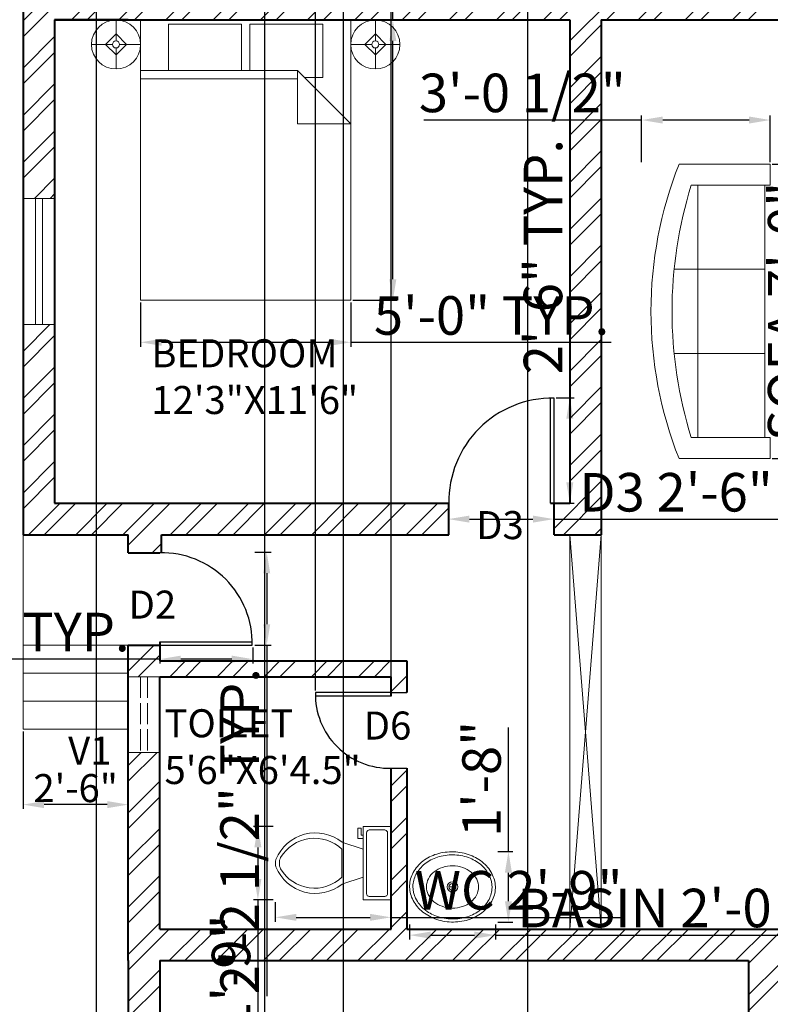
# Model space of a CAD drawing. Units: inches. Extents: x 2069 to 3028, y 691 to 1726.
# Tile 4 of 10: x 2267 to 2481, y 1044 to 1325. Entities that reach past the tile are written whole.
import ezdxf

# ---------------------------------------------------------------- set-up
doc = ezdxf.new("R2010")
doc.units = ezdxf.units.IN
doc.linetypes.add('ACAD_ISO02W100', pattern=[15, 12, -3])
for name, color, linetype, lineweight in [('A-ANNO-DIMS', 2, 'Continuous', 18), ('A-DOOR', 3, 'Continuous', 25), ('A-FLOR-FIXT', 9, 'Continuous', 20), ('A-FLOR-STRS', 7, 'Continuous', 20), ('A-FURN', 8, 'Continuous', 18), ('A-GLAZ', 4, 'Continuous', 20), ('A-GLAZ-HIDN', 4, 'ACAD_ISO02W100', 18), ('A-WALL', 7, 'Continuous', 40)]:
    doc.layers.add(name, color=color, linetype=linetype, lineweight=lineweight)
for name, color, linetype, lineweight, true_color in [('A-ANNO-TEXT', 11, 'Continuous', 18, 0xf27172), ('A-AREA-IDEN', 11, 'Continuous', 25, 0xf27172), ('A-WALL-OPEN', 143, 'Continuous', 20, 0x7aafdf), ('A-WALL-PATT', 143, 'Continuous', 13, 0x7aafdf)]:
    doc.layers.add(name, color=color, linetype=linetype, lineweight=lineweight, true_color=true_color)
doc.styles.get("Standard").update_dxf_attribs({"font": 'arial.ttf'})
doc.dimstyles.new('ISO-25', dxfattribs={"dimtxt": 11, "dimasz": 6, "dimexe": 1.25, "dimexo": 0.625, "dimtad": 1, "dimlunit": 3, "dimtxsty": 'Standard', "dimcen": 2.5, "dimclrd": 3, "dimclre": 5, "dimclrt": 6, "dimadec": 0, "dimazin": 0, "dimtfac": 1, "dimtmove": 0, "dimatfit": 3, "dimfxl": 1, "dimarcsym": 0})

# ---------------------------------------------------------------- blocks, each defined once
blk = doc.blocks.new('Sink - Oval top')
for p, q in [((-1, 0), (1, 0)), ((0, 1), (0, -1))]:
    blk.add_line(p, q)
for points in [[(-12.23, 0.39, 0.117634), (-11.46, -3.36, 0.104469), (-8.88, -6.8, 0.090016), (-5.08, -9.07, 0.08192), (-0.32, -10.02, 0.08192), (4.49, -9.38, 0.090016), (8.42, -7.36, 0.104469), (11.22, -4.09, 0.117634), (12.23, -0.39, 0.117634), (11.46, 3.36, 0.104469), (8.88, 6.8, 0.090016), (5.08, 9.07, 0.08192), (0.32, 10.02, 0.08192), (-4.49, 9.38, 0.090016), (-8.42, 7.36, 0.104469), (-11.22, 4.09, 0.117634)], [(-11.29, 0.16, 0.118622), (-10.52, -3.25, 0.104678), (-8.07, -6.36, 0.089562), (-4.54, -8.37, 0.081185), (-0.13, -9.15, 0.081185), (4.3, -8.49, 0.089562), (7.89, -6.58, 0.104678), (10.42, -3.55, 0.118622), (11.29, -0.16, 0.118622), (10.52, 3.25, 0.104678), (8.07, 6.36, 0.089562), (4.54, 8.37, 0.081185), (0.13, 9.15, 0.081185), (-4.3, 8.49, 0.089562), (-7.89, 6.58, 0.104678), (-10.42, 3.55, 0.118622)], [(-7.42, 0.08, 0.118283), (-6.91, -2.17, 0.104607), (-5.29, -4.21, 0.089718), (-2.97, -5.53, 0.081436), (-0.07, -6.04, 0.081436), (2.84, -5.59, 0.089718), (5.2, -4.33, 0.104607), (6.86, -2.32, 0.118283), (7.42, -0.08, 0.118283), (6.91, 2.17, 0.104607), (5.29, 4.21, 0.089718), (2.97, 5.53, 0.081436), (0.07, 6.04, 0.081436), (-2.84, 5.59, 0.089718), (-5.2, 4.33, 0.104607), (-6.86, 2.32, 0.118283)]]:
    blk.add_lwpolyline(points, format="xyb", close=True)
for radius in [1.5, 1]:
    blk.add_circle((0, 0), radius)
blk = doc.blocks.new('Bed - Queen')
for p, q in [((0, -80.00003), (0, 0)), ((0, 0), (59.99999, 0)), ((59.99999, 0), (59.99999, -80.00003)), ((7.99999, -1.2), (28.79998, -1.2)), ((7.99999, -14.4), (7.99999, -1.2)), ((28.79998, -1.2), (28.79998, -14.4)), ((31.19999, -1.2), (51.99999, -1.2)), ((31.19999, -14.4), (31.19999, -1.2)), ((51.99999, -1.2), (51.99999, -16.4)), ((0, -14.4), (44.8, -14.4)), ((44.8, -16.8), (0, -16.8)), ((59.99999, -29.6), (44.8, -14.4)), ((44.8, -14.4), (44.8, -29.6)), ((51.99999, -16.4), (46.79936, -16.4)), ((44.8, -29.6), (59.99999, -29.6)), ((59.99999, -80.00003), (0, -80.00003))]:
    blk.add_line(p, q)
blk = doc.blocks.new('Lamp - Table')
for p, q in [((0, 7), (0, 1)), ((0, 3), (-3, 0)), ((3, 0), (0, 3)), ((-1, 0), (-7, 0)), ((-3, 0), (0, -3)), ((0, -3), (3, 0)), ((1, 0), (7, 0)), ((0, -1), (0, -7))]:
    blk.add_line(p, q)
for radius in [7, 1]:
    blk.add_circle((0, 0), radius)
blk = doc.blocks.new('Sofa - Roundback 7 ft.')
for p, q in [((-12.00002, -32.4421), (-12.00003, -6.5971)), ((11.99997, -32.4421), (11.99998, -6.5971)), ((-36.000027, -34), (-36.000027, -11.4696)), ((-35.999844, -13.3819), (35.9998, -13.3819)), ((35.99998, -34), (35.99998, -11.4696)), ((-36.000027, -32.4421), (35.99998, -32.4421))]:
    blk.add_line(p, q)
for points in [[(-36.000027, -34), (-42.000027, -34), (-42.000027, -8)], [(41.99998, -8), (41.99998, -34), (35.99998, -34)]]:
    blk.add_lwpolyline(points)
for centre, radius, start, end in [((0, -114.25), 114.25, 68.43141, 111.5686), ((-0.00001, -127.1968), 121.1968, 72.72033, 107.2797)]:
    blk.add_arc(centre, radius, start, end)
blk = doc.blocks.new('Toilet - top')
for p, q in [((9.5, -6), (9.5, -2)), ((-8, -8.5), (-8, -8)), ((-7, -8), (-7, -9.5)), ((-4, -8), (-6, -14)), ((4, -8), (6, -14)), ((-10, -8.5), (-8, -8.5)), ((-10, -9.5), (-10, -8.5)), ((-7, -9.5), (-10, -9.5)), ((4, -14), (-4, -14))]:
    blk.add_line(p, q)
blk.add_lwpolyline([(10.5, -8), (10.5, 0), (-10.5, 0), (-10.5, -8)], close=True)
for points in [[(-9.5, -2), (-9.5, -6)], [(8.5, -1), (-8.5, -1)], [(-8.5, -7), (8.5, -7)]]:
    blk.add_lwpolyline(points)
for centre, radius, start, end in [((-8.62, -1.88), 0.884, 81.8699, 188.1301), ((8.62, -1.88), 0.884, 351.8699, 98.1301), ((-8.62, -6.12), 0.884, 171.8699, 278.1301), ((8.62, -6.12), 0.884, 261.8699, 8.1301), ((3.52, -21.58), 12.17, 141.4691, 247.9714), ((4.2, -21.82), 11.33, 136.3677, 238.9468), ((-3.52, -21.58), 12.17, 292.0284, 38.5307), ((-4.2, -21.82), 11.33, 301.053, 43.6321), ((0, -27.88), 4, 245.7318, 294.2682), ((0, -29), 4, 254.8605, 285.1395)]:
    blk.add_arc(centre, radius, start, end)
blk = doc.blocks.new('*D33')
at = {"layer": 'A-ANNO-DIMS', "color": 0, "lineweight": -2, "transparency": 16777216}
for p, q in [((2267.95, 1122.26), (2267.95, 1100.15)), ((2297.95, 1122.26), (2297.95, 1100.15)), ((2291.95, 1101.4), (2273.95, 1101.4))]:
    blk.add_line(p, q, dxfattribs=at)
at = {"layer": 'A-ANNO-DIMS', "color": 0, "transparency": 16777216}
for points in [[(2273.95, 1102.4), (2273.95, 1100.4), (2267.95, 1101.4)], [(2291.95, 1102.4), (2291.95, 1100.4), (2297.95, 1101.4)]]:
    blk.add_solid(points, dxfattribs=at)
at = {"layer": 'Defpoints', "color": 0, "transparency": 16777216}
for p in [(2267.95, 1122.89), (2297.95, 1122.89), (2267.95, 1101.4)]:
    blk.add_point(p, dxfattribs=at)
at = {"layer": 'A-ANNO-DIMS', "color": 0, "transparency": 16777216, "insert": (2282.95, 1106.11), "char_height": 11, "width": 27.3807, "attachment_point": 5}
blk.add_mtext('{\\H0.72727x;2\'-6"}', dxfattribs=at)
blk = doc.blocks.new('DOOR-SWING-26_4IN')
for p, q in [((0, 0), (-26.4, 0)), ((0, -1), (-26.4, -1))]:
    blk.add_line(p, q)
blk.add_arc((-0.5, -0.5), 25.9, 178.894, 271.106)
blk = doc.blocks.new('DOOR-SWING-30IN')
for p, q in [((-1, 0), (-1, 30)), ((0, 0), (0, 30))]:
    blk.add_line(p, q)
blk.add_arc((-0.5, 0.5), 29.5, 89.029, 180.971)
blk = doc.blocks.new('WINDOW-36IN')
for p, q in [((0, 0), (9, 0)), ((3.5, 0), (3.5, -36)), ((5.5, 0), (5.5, -36)), ((0, -36), (9, -36))]:
    blk.add_line(p, q)
blk = doc.blocks.new('CASED-OPENING-112_5IN')
for p, q in [((9, 0), (0, -112.5)), ((9, -112.5), (0, 0)), ((0, 0), (0, -112.5)), ((9, 0), (9, -112.5))]:
    blk.add_line(p, q)
blk = doc.blocks.new('*D54')
at = {"layer": 'A-ANNO-DIMS', "color": 3, "lineweight": -2, "transparency": 16777216}
for p, q in [((2373.46, 1325.32), (2373.46, 1494.38)), ((2373.46, 1251.32), (2373.46, 1319.32))]:
    blk.add_line(p, q, dxfattribs=at)
at = {"layer": 'A-ANNO-DIMS', "color": 5, "lineweight": -2, "transparency": 16777216}
for p, q in [((2362.09, 1325.32), (2374.71, 1325.32)), ((2362.09, 1245.32), (2374.71, 1245.32))]:
    blk.add_line(p, q, dxfattribs=at)
at = {"layer": 'A-ANNO-DIMS', "color": 3, "transparency": 16777216}
for points in [[(2372.46, 1319.32), (2374.46, 1319.32), (2373.46, 1325.32)], [(2372.46, 1251.32), (2374.46, 1251.32), (2373.46, 1245.32)]]:
    blk.add_solid(points, dxfattribs=at)
at = {"layer": 'Defpoints', "color": 0, "transparency": 16777216}
for p in [(2361.46, 1325.32), (2373.46, 1325.32), (2361.46, 1245.32)]:
    blk.add_point(p, dxfattribs=at)
at = {"layer": 'A-ANNO-DIMS', "color": 6, "transparency": 16777216, "insert": (2366.81, 1412.85), "char_height": 11, "attachment_point": 5, "rotation": 90}
blk.add_mtext('QUEEN BED 6\'-8" TYP.', dxfattribs=at)
blk = doc.blocks.new('*D55')
at = {"layer": 'A-ANNO-DIMS', "color": 5, "lineweight": -2, "transparency": 16777216}
for p, q in [((2301.46, 1244.69), (2301.46, 1232.07)), ((2361.46, 1244.69), (2361.46, 1232.07))]:
    blk.add_line(p, q, dxfattribs=at)
at = {"layer": 'A-ANNO-DIMS', "color": 3, "lineweight": -2, "transparency": 16777216}
for p, q in [((2307.46, 1233.32), (2355.46, 1233.32)), ((2361.46, 1233.32), (2435.77, 1233.32))]:
    blk.add_line(p, q, dxfattribs=at)
at = {"layer": 'A-ANNO-DIMS', "color": 3, "transparency": 16777216}
for points in [[(2307.46, 1234.32), (2307.46, 1232.32), (2301.46, 1233.32)], [(2355.46, 1234.32), (2355.46, 1232.32), (2361.46, 1233.32)]]:
    blk.add_solid(points, dxfattribs=at)
at = {"layer": 'Defpoints', "color": 0, "transparency": 16777216}
for p in [(2301.46, 1245.32), (2361.46, 1245.32), (2361.46, 1233.32)]:
    blk.add_point(p, dxfattribs=at)
at = {"layer": 'A-ANNO-DIMS', "color": 6, "transparency": 16777216, "insert": (2401.62, 1239.56), "char_height": 11, "attachment_point": 5}
blk.add_mtext('5\'-0" TYP.', dxfattribs=at)
blk = doc.blocks.new('*D56')
at = {"layer": 'A-ANNO-DIMS', "color": 5, "lineweight": -2, "transparency": 16777216}
for p, q in [((2389.32, 1186.76), (2389.32, 1181.62)), ((2419.45, 1186.76), (2419.45, 1181.62))]:
    blk.add_line(p, q, dxfattribs=at)
at = {"layer": 'A-ANNO-DIMS', "color": 3, "lineweight": -2, "transparency": 16777216}
for p, q in [((2395.32, 1182.87), (2413.45, 1182.87)), ((2419.45, 1182.87), (2517.12, 1182.87))]:
    blk.add_line(p, q, dxfattribs=at)
at = {"layer": 'A-ANNO-DIMS', "color": 3, "transparency": 16777216}
for points in [[(2395.32, 1183.87), (2395.32, 1181.87), (2389.32, 1182.87)], [(2413.45, 1183.87), (2413.45, 1181.87), (2419.45, 1182.87)]]:
    blk.add_solid(points, dxfattribs=at)
at = {"layer": 'Defpoints', "color": 0, "transparency": 16777216}
for p in [(2389.32, 1187.39), (2419.45, 1187.39), (2419.45, 1182.87)]:
    blk.add_point(p, dxfattribs=at)
at = {"layer": 'A-ANNO-DIMS', "color": 6, "transparency": 16777216, "insert": (2471.28, 1189.11), "char_height": 11, "attachment_point": 5}
blk.add_mtext('D3 2\'-6" TYP.', dxfattribs=at)
blk = doc.blocks.new('*D57')
at = {"layer": 'A-ANNO-DIMS', "color": 3, "lineweight": -2, "transparency": 16777216}
for p, q in [((2423.97, 1217.52), (2423.97, 1292.01)), ((2423.97, 1193.39), (2423.97, 1211.52))]:
    blk.add_line(p, q, dxfattribs=at)
at = {"layer": 'A-ANNO-DIMS', "color": 5, "lineweight": -2, "transparency": 16777216}
for p, q in [((2420.08, 1217.52), (2425.22, 1217.52)), ((2420.08, 1187.39), (2425.22, 1187.39))]:
    blk.add_line(p, q, dxfattribs=at)
at = {"layer": 'A-ANNO-DIMS', "color": 3, "transparency": 16777216}
for points in [[(2422.97, 1211.52), (2424.97, 1211.52), (2423.97, 1217.52)], [(2422.97, 1193.39), (2424.97, 1193.39), (2423.97, 1187.39)]]:
    blk.add_solid(points, dxfattribs=at)
at = {"layer": 'Defpoints', "color": 0, "transparency": 16777216}
for p in [(2419.45, 1217.52), (2423.97, 1217.52), (2419.45, 1187.39)]:
    blk.add_point(p, dxfattribs=at)
at = {"layer": 'A-ANNO-DIMS', "color": 6, "transparency": 16777216, "insert": (2417.73, 1257.77), "char_height": 11, "attachment_point": 5, "rotation": 90}
blk.add_mtext('2\'-6" TYP.', dxfattribs=at)
blk = doc.blocks.new('*D64')
at = {"layer": 'A-ANNO-DIMS', "color": 5, "lineweight": -2, "transparency": 16777216}
for p, q in [((2306.95, 1146.26), (2306.95, 1141.66)), ((2333.49, 1146.26), (2333.49, 1141.66))]:
    blk.add_line(p, q, dxfattribs=at)
at = {"layer": 'A-ANNO-DIMS', "color": 3, "lineweight": -2, "transparency": 16777216}
for p, q in [((2306.95, 1142.91), (2157.2, 1142.91)), ((2327.49, 1142.91), (2312.95, 1142.91))]:
    blk.add_line(p, q, dxfattribs=at)
at = {"layer": 'A-ANNO-DIMS', "color": 3, "transparency": 16777216}
for points in [[(2312.95, 1143.91), (2312.95, 1141.91), (2306.95, 1142.91)], [(2327.49, 1143.91), (2327.49, 1141.91), (2333.49, 1142.91)]]:
    blk.add_solid(points, dxfattribs=at)
at = {"layer": 'Defpoints', "color": 0, "transparency": 16777216}
for p in [(2306.95, 1146.89), (2333.49, 1146.89), (2306.95, 1142.91)]:
    blk.add_point(p, dxfattribs=at)
at = {"layer": 'A-ANNO-DIMS', "color": 6, "transparency": 16777216, "insert": (2229.07, 1149.22), "char_height": 11, "attachment_point": 5}
blk.add_mtext('DOOR 2\'-2 1/2" TYP.', dxfattribs=at)
blk = doc.blocks.new('*D65')
at = {"layer": 'A-ANNO-DIMS', "color": 5, "lineweight": -2, "transparency": 16777216}
for p, q in [((2334.11, 1173.42), (2338.72, 1173.42)), ((2334.11, 1146.89), (2338.72, 1146.89))]:
    blk.add_line(p, q, dxfattribs=at)
at = {"layer": 'A-ANNO-DIMS', "color": 3, "lineweight": -2, "transparency": 16777216}
for p, q in [((2337.47, 1167.42), (2337.47, 1152.89)), ((2337.47, 1146.89), (2337.47, 1046.77))]:
    blk.add_line(p, q, dxfattribs=at)
at = {"layer": 'A-ANNO-DIMS', "color": 3, "transparency": 16777216}
for points in [[(2336.47, 1167.42), (2338.47, 1167.42), (2337.47, 1173.42)], [(2336.47, 1152.89), (2338.47, 1152.89), (2337.47, 1146.89)]]:
    blk.add_solid(points, dxfattribs=at)
at = {"layer": 'Defpoints', "color": 0, "transparency": 16777216}
for p in [(2333.49, 1173.42), (2333.49, 1146.89), (2337.47, 1146.89)]:
    blk.add_point(p, dxfattribs=at)
at = {"layer": 'A-ANNO-DIMS', "color": 6, "transparency": 16777216, "insert": (2331.16, 1093.83), "char_height": 11, "attachment_point": 5, "rotation": 90}
blk.add_mtext('2\'-2 1/2" TYP.', dxfattribs=at)
blk = doc.blocks.new('*D76')
at = {"layer": 'A-ANNO-DIMS', "color": 5, "lineweight": -2, "transparency": 16777216}
for p, q in [((2378.21, 1067.22), (2378.21, 1062.91)), ((2402.76, 1067.22), (2402.76, 1062.91))]:
    blk.add_line(p, q, dxfattribs=at)
at = {"layer": 'A-ANNO-DIMS', "color": 3, "lineweight": -2, "transparency": 16777216}
for p, q in [((2384.21, 1064.16), (2396.76, 1064.16)), ((2402.76, 1064.16), (2514.78, 1064.16))]:
    blk.add_line(p, q, dxfattribs=at)
at = {"layer": 'A-ANNO-DIMS', "color": 3, "transparency": 16777216}
for points in [[(2384.21, 1065.16), (2384.21, 1063.16), (2378.21, 1064.16)], [(2396.76, 1065.16), (2396.76, 1063.16), (2402.76, 1064.16)]]:
    blk.add_solid(points, dxfattribs=at)
at = {"layer": 'Defpoints', "color": 0, "transparency": 16777216}
for p in [(2378.21, 1067.84), (2402.76, 1067.84), (2402.76, 1064.16)]:
    blk.add_point(p, dxfattribs=at)
at = {"layer": 'A-ANNO-DIMS', "color": 6, "transparency": 16777216, "insert": (2461.77, 1070.47), "char_height": 11, "attachment_point": 5}
blk.add_mtext('BASIN 2\'-0 1/2"', dxfattribs=at)
blk = doc.blocks.new('*D77')
at = {"layer": 'A-ANNO-DIMS', "color": 3, "lineweight": -2, "transparency": 16777216}
for p, q in [((2406.44, 1087.98), (2406.44, 1123.44)), ((2406.44, 1073.84), (2406.44, 1081.98))]:
    blk.add_line(p, q, dxfattribs=at)
at = {"layer": 'A-ANNO-DIMS', "color": 5, "lineweight": -2, "transparency": 16777216}
for p, q in [((2403.38, 1087.98), (2407.69, 1087.98)), ((2403.38, 1067.84), (2407.69, 1067.84))]:
    blk.add_line(p, q, dxfattribs=at)
at = {"layer": 'A-ANNO-DIMS', "color": 3, "transparency": 16777216}
for points in [[(2405.44, 1081.98), (2407.44, 1081.98), (2406.44, 1087.98)], [(2405.44, 1073.84), (2407.44, 1073.84), (2406.44, 1067.84)]]:
    blk.add_solid(points, dxfattribs=at)
at = {"layer": 'Defpoints', "color": 0, "transparency": 16777216}
for p in [(2402.76, 1087.98), (2406.44, 1087.98), (2402.76, 1067.84)]:
    blk.add_point(p, dxfattribs=at)
at = {"layer": 'A-ANNO-DIMS', "color": 6, "transparency": 16777216, "insert": (2400.2, 1108.71), "char_height": 11, "attachment_point": 5, "rotation": 90}
blk.add_mtext('1\'-8"', dxfattribs=at)
blk = doc.blocks.new('*D82')
at = {"layer": 'A-ANNO-DIMS', "color": 5, "lineweight": -2, "transparency": 16777216}
for p, q in [((2481.75, 1284.15), (2494.98, 1284.15)), ((2481.75, 1200.15), (2494.98, 1200.15))]:
    blk.add_line(p, q, dxfattribs=at)
at = {"layer": 'A-ANNO-DIMS', "color": 3, "lineweight": -2, "transparency": 16777216}
blk.add_line((2493.73, 1206.15), (2493.73, 1278.15), dxfattribs=at)
at = {"layer": 'A-ANNO-DIMS', "color": 3, "transparency": 16777216}
for points in [[(2492.73, 1278.15), (2494.73, 1278.15), (2493.73, 1284.15)], [(2492.73, 1206.15), (2494.73, 1206.15), (2493.73, 1200.15)]]:
    blk.add_solid(points, dxfattribs=at)
at = {"layer": 'Defpoints', "color": 0, "transparency": 16777216}
for p in [(2481.13, 1284.15), (2493.73, 1284.15), (2481.13, 1200.15)]:
    blk.add_point(p, dxfattribs=at)
at = {"layer": 'A-ANNO-DIMS', "color": 6, "transparency": 16777216, "insert": (2487.41, 1242.15), "char_height": 11, "attachment_point": 5, "rotation": 90}
blk.add_mtext('SOFA 7\'-0"', dxfattribs=at)
blk = doc.blocks.new('*D83')
at = {"layer": 'A-ANNO-DIMS', "color": 3, "lineweight": -2, "transparency": 16777216}
for p, q in [((2444.46, 1296.75), (2382.34, 1296.75)), ((2475.13, 1296.75), (2450.46, 1296.75))]:
    blk.add_line(p, q, dxfattribs=at)
at = {"layer": 'A-ANNO-DIMS', "color": 5, "lineweight": -2, "transparency": 16777216}
for p, q in [((2444.46, 1284.77), (2444.46, 1298)), ((2481.13, 1284.77), (2481.13, 1298))]:
    blk.add_line(p, q, dxfattribs=at)
at = {"layer": 'A-ANNO-DIMS', "color": 3, "transparency": 16777216}
for points in [[(2450.46, 1297.75), (2450.46, 1295.75), (2444.46, 1296.75)], [(2475.13, 1297.75), (2475.13, 1295.75), (2481.13, 1296.75)]]:
    blk.add_solid(points, dxfattribs=at)
at = {"layer": 'Defpoints', "color": 0, "transparency": 16777216}
for p in [(2444.46, 1296.75), (2444.46, 1284.15), (2481.13, 1284.15)]:
    blk.add_point(p, dxfattribs=at)
at = {"layer": 'A-ANNO-DIMS', "color": 6, "transparency": 16777216, "insert": (2410.4, 1303.07), "char_height": 11, "attachment_point": 5}
blk.add_mtext('3\'-0 1/2"', dxfattribs=at)
blk = doc.blocks.new('*D84')
at = {"layer": 'A-ANNO-DIMS', "color": 5, "lineweight": -2, "transparency": 16777216}
for p, q in [((2339.91, 1073.56), (2339.91, 1067.98)), ((2372.95, 1073.56), (2372.95, 1067.98))]:
    blk.add_line(p, q, dxfattribs=at)
at = {"layer": 'A-ANNO-DIMS', "color": 3, "lineweight": -2, "transparency": 16777216}
for p, q in [((2345.91, 1069.23), (2366.95, 1069.23)), ((2372.95, 1069.23), (2439.76, 1069.23))]:
    blk.add_line(p, q, dxfattribs=at)
at = {"layer": 'A-ANNO-DIMS', "color": 3, "transparency": 16777216}
for points in [[(2345.91, 1070.23), (2345.91, 1068.23), (2339.91, 1069.23)], [(2366.95, 1070.23), (2366.95, 1068.23), (2372.95, 1069.23)]]:
    blk.add_solid(points, dxfattribs=at)
at = {"layer": 'Defpoints', "color": 0, "transparency": 16777216}
for p in [(2339.91, 1074.19), (2372.95, 1074.19), (2372.95, 1069.23)]:
    blk.add_point(p, dxfattribs=at)
at = {"layer": 'A-ANNO-DIMS', "color": 6, "transparency": 16777216, "insert": (2409.36, 1075.54), "char_height": 11, "attachment_point": 5}
blk.add_mtext('WC 2\'-9"', dxfattribs=at)
blk = doc.blocks.new('*D85')
at = {"layer": 'A-ANNO-DIMS', "color": 5, "lineweight": -2, "transparency": 16777216}
for p, q in [((2339.28, 1095.19), (2333.7, 1095.19)), ((2339.28, 1074.19), (2333.7, 1074.19))]:
    blk.add_line(p, q, dxfattribs=at)
at = {"layer": 'A-ANNO-DIMS', "color": 3, "lineweight": -2, "transparency": 16777216}
for p, q in [((2334.95, 1089.19), (2334.95, 1080.19)), ((2334.95, 1074.19), (2334.95, 1038.73))]:
    blk.add_line(p, q, dxfattribs=at)
at = {"layer": 'A-ANNO-DIMS', "color": 3, "transparency": 16777216}
for points in [[(2333.95, 1089.19), (2335.95, 1089.19), (2334.95, 1095.19)], [(2333.95, 1080.19), (2335.95, 1080.19), (2334.95, 1074.19)]]:
    blk.add_solid(points, dxfattribs=at)
at = {"layer": 'Defpoints', "color": 0, "transparency": 16777216}
for p in [(2339.91, 1095.19), (2334.95, 1074.19), (2339.91, 1074.19)]:
    blk.add_point(p, dxfattribs=at)
at = {"layer": 'A-ANNO-DIMS', "color": 6, "transparency": 16777216, "insert": (2328.71, 1053.46), "char_height": 11, "attachment_point": 5, "rotation": 90}
blk.add_mtext('1\'-9"', dxfattribs=at)
blk = doc.blocks.new('*D87')
at = {"layer": 'A-ANNO-DIMS', "color": 5, "lineweight": -2, "transparency": 16777216}
for p, q in [((2297.33, 1487.39), (2090.2, 1487.39)), ((2297.33, 903.89), (2090.2, 903.89))]:
    blk.add_line(p, q, dxfattribs=at)
at = {"layer": 'A-ANNO-DIMS', "color": 3, "lineweight": -2, "transparency": 16777216}
blk.add_line((2091.45, 909.89), (2091.45, 1481.39), dxfattribs=at)
at = {"layer": 'A-ANNO-DIMS', "color": 3, "transparency": 16777216}
for points in [[(2090.45, 1481.39), (2092.45, 1481.39), (2091.45, 1487.39)], [(2090.45, 909.89), (2092.45, 909.89), (2091.45, 903.89)]]:
    blk.add_solid(points, dxfattribs=at)
at = {"layer": 'Defpoints', "color": 0, "transparency": 16777216}
for p in [(2091.45, 1487.39), (2297.95, 1487.39), (2297.95, 903.89)]:
    blk.add_point(p, dxfattribs=at)
at = {"layer": 'A-ANNO-DIMS', "color": 6, "transparency": 16777216, "insert": (2085.14, 1195.64), "char_height": 11, "attachment_point": 5, "rotation": 90}
blk.add_mtext('48\'-7 1/2"', dxfattribs=at)
blk = doc.blocks.new('*D88')
at = {"layer": 'A-ANNO-DIMS', "color": 5, "lineweight": -2, "transparency": 16777216}
for p, q in [((2288.92, 738.01), (2288.92, 1704.14)), ((2336.92, 738.01), (2336.92, 1704.14))]:
    blk.add_line(p, q, dxfattribs=at)
at = {"layer": 'A-ANNO-DIMS', "color": 3, "lineweight": -2, "transparency": 16777216}
blk.add_line((2294.92, 1702.89), (2330.92, 1702.89), dxfattribs=at)
at = {"layer": 'A-ANNO-DIMS', "color": 3, "transparency": 16777216}
for points in [[(2294.92, 1703.89), (2294.92, 1701.89), (2288.92, 1702.89)], [(2330.92, 1703.89), (2330.92, 1701.89), (2336.92, 1702.89)]]:
    blk.add_solid(points, dxfattribs=at)
at = {"layer": 'Defpoints', "color": 0, "transparency": 16777216}
for p in [(2336.92, 1702.89), (2288.92, 737.39), (2336.92, 737.39)]:
    blk.add_point(p, dxfattribs=at)
at = {"layer": 'A-ANNO-DIMS', "color": 6, "transparency": 16777216, "insert": (2312.92, 1709.13), "char_height": 11, "attachment_point": 5}
blk.add_mtext('4\'-0"', dxfattribs=at)
blk = doc.blocks.new('*D89')
at = {"layer": 'A-ANNO-DIMS', "color": 5, "lineweight": -2, "transparency": 16777216}
for p, q in [((2336.92, 747.01), (2336.92, 1704.14)), ((2711.95, 747.01), (2711.95, 1704.14))]:
    blk.add_line(p, q, dxfattribs=at)
at = {"layer": 'A-ANNO-DIMS', "color": 3, "lineweight": -2, "transparency": 16777216}
blk.add_line((2342.92, 1702.89), (2705.95, 1702.89), dxfattribs=at)
at = {"layer": 'A-ANNO-DIMS', "color": 3, "transparency": 16777216}
for points in [[(2342.92, 1703.89), (2342.92, 1701.89), (2336.92, 1702.89)], [(2705.95, 1703.89), (2705.95, 1701.89), (2711.95, 1702.89)]]:
    blk.add_solid(points, dxfattribs=at)
at = {"layer": 'Defpoints', "color": 0, "transparency": 16777216}
for p in [(2711.95, 1702.89), (2336.92, 746.39), (2711.95, 746.39)]:
    blk.add_point(p, dxfattribs=at)
at = {"layer": 'A-ANNO-DIMS', "color": 6, "transparency": 16777216, "insert": (2524.44, 1709.13), "char_height": 11, "attachment_point": 5}
blk.add_mtext('31\'-3"', dxfattribs=at)
blk = doc.blocks.new('*D92')
at = {"layer": 'A-ANNO-DIMS', "color": 5, "lineweight": -2, "transparency": 16777216}
for p, q in [((2359.37, 992.45), (2359.37, 1704.14)), ((2411.94, 992.45), (2411.94, 1704.14))]:
    blk.add_line(p, q, dxfattribs=at)
at = {"layer": 'A-ANNO-DIMS', "color": 3, "lineweight": -2, "transparency": 16777216}
for p, q in [((2365.37, 1702.89), (2405.94, 1702.89)), ((2411.94, 1702.89), (2474.5, 1702.89))]:
    blk.add_line(p, q, dxfattribs=at)
at = {"layer": 'A-ANNO-DIMS', "color": 3, "transparency": 16777216}
for points in [[(2365.37, 1703.89), (2365.37, 1701.89), (2359.37, 1702.89)], [(2405.94, 1703.89), (2405.94, 1701.89), (2411.94, 1702.89)]]:
    blk.add_solid(points, dxfattribs=at)
at = {"layer": 'Defpoints', "color": 0, "transparency": 16777216}
for p in [(2411.94, 1702.89), (2359.37, 991.83), (2411.94, 991.83)]:
    blk.add_point(p, dxfattribs=at)
at = {"layer": 'A-ANNO-DIMS', "color": 6, "transparency": 16777216, "insert": (2446.22, 1709.2), "char_height": 11, "attachment_point": 5}
blk.add_mtext('4\'-4 1/2"', dxfattribs=at)
blk = doc.blocks.new('*D95')
at = {"layer": 'A-ANNO-DIMS', "color": 5, "lineweight": -2, "transparency": 16777216}
for p, q in [((2351.35, 1134.01), (2351.35, 1704.14)), ((2372.95, 1134.01), (2372.95, 1704.14))]:
    blk.add_line(p, q, dxfattribs=at)
at = {"layer": 'A-ANNO-DIMS', "color": 3, "lineweight": -2, "transparency": 16777216}
for p, q in [((2357.35, 1702.89), (2366.95, 1702.89)), ((2372.95, 1702.89), (2434.04, 1702.89))]:
    blk.add_line(p, q, dxfattribs=at)
at = {"layer": 'A-ANNO-DIMS', "color": 3, "transparency": 16777216}
for points in [[(2357.35, 1703.89), (2357.35, 1701.89), (2351.35, 1702.89)], [(2366.95, 1703.89), (2366.95, 1701.89), (2372.95, 1702.89)]]:
    blk.add_solid(points, dxfattribs=at)
at = {"layer": 'Defpoints', "color": 0, "transparency": 16777216}
for p in [(2372.95, 1702.89), (2351.35, 1133.39), (2372.95, 1133.39)]:
    blk.add_point(p, dxfattribs=at)
at = {"layer": 'A-ANNO-DIMS', "color": 6, "transparency": 16777216, "insert": (2406.49, 1709.2), "char_height": 11, "attachment_point": 5}
blk.add_mtext('1\'-9 1/2"', dxfattribs=at)

msp = doc.modelspace()

# ---------------------------------------------------------------- hatches: boundary and pattern name
at = {"layer": 'A-WALL-PATT'}
h = msp.add_hatch(dxfattribs=at)
h.set_pattern_fill('ANSI32', color=256)
h.paths.add_polyline_path([(2675.951, 1487.387), (2576.951, 1487.387), (2576.951, 1478.387), (2621.951, 1478.387), (2621.951, 1365.287), (2630.951, 1365.287), (2630.951, 1478.387), (2675.951, 1478.387)])
h.paths.add_polyline_path([(2765.951, 1487.387), (2711.951, 1487.387), (2711.951, 1478.387), (2756.951, 1478.387), (2756.951, 1424.387), (2765.951, 1424.387)])
h.paths.add_polyline_path([(2528.951, 1487.387), (2407.751, 1487.387), (2407.751, 1478.387), (2474.951, 1478.387), (2474.951, 1434.887), (2498.951, 1434.887), (2498.951, 1374.887), (2474.951, 1374.887), (2474.951, 1365.287), (2483.951, 1365.287), (2483.951, 1370.387), (2507.951, 1370.387), (2507.951, 1439.387), (2483.951, 1439.387), (2483.951, 1478.387), (2528.951, 1478.387)])
h.paths.add_polyline_path([(2374.151, 1487.387), (2297.951, 1487.387), (2297.951, 1424.387), (2306.951, 1424.387), (2306.951, 1478.387), (2374.151, 1478.387)])
h.paths.add_polyline_path([(2507.951, 1334.387), (2483.951, 1334.387), (2483.951, 1338.887), (2474.951, 1338.887), (2474.951, 1334.387), (2306.951, 1334.387), (2306.951, 1388.387), (2297.951, 1388.387), (2297.951, 1334.387), (2267.951, 1334.387), (2267.951, 1274.387), (2276.951, 1274.387), (2276.951, 1325.387), (2297.951, 1325.387), (2423.951, 1325.387), (2423.951, 1187.387), (2419.451, 1187.387), (2419.451, 1178.387), (2432.951, 1178.387), (2432.951, 1325.387), (2507.951, 1325.387)])
h.paths.add_polyline_path([(2795.951, 1334.387), (2630.951, 1334.387), (2630.951, 1338.887), (2621.951, 1338.887), (2621.951, 1178.387), (2635.451, 1178.387), (2635.451, 1187.387), (2630.951, 1187.387), (2630.951, 1325.387), (2786.951, 1325.387), (2786.951, 1274.387), (2795.951, 1274.387)])
h.paths.add_polyline_path([(2765.951, 1388.387), (2756.951, 1388.387), (2756.951, 1334.387), (2765.951, 1334.387)])
h.paths.add_polyline_path([(2795.951, 1238.387), (2786.951, 1238.387), (2786.951, 1187.387), (2665.451, 1187.387), (2665.451, 1178.387), (2795.951, 1178.387)], flags=17)
h.paths.add_polyline_path([(2389.451, 1187.387), (2276.951, 1187.387), (2276.951, 1238.387), (2267.951, 1238.387), (2267.951, 1178.387), (2297.951, 1178.387), (2297.951, 1173.287), (2307.451, 1173.287), (2307.451, 1178.387), (2389.451, 1178.387)])
h.paths.add_polyline_path([(2377.451, 1142.387), (2306.951, 1142.387), (2306.951, 1146.887), (2297.951, 1146.887), (2297.951, 1142.387), (2297.951, 1137.887), (2306.951, 1137.887), (2372.951, 1137.887), (2372.951, 1133.387), (2377.451, 1133.387)])
h.paths.add_polyline_path([(2795.951, 1065.887), (2665.451, 1065.887), (2665.451, 1056.887), (2786.951, 1056.887), (2786.951, 1002.887), (2795.951, 1002.887), (2795.951, 1056.887)])
h.paths.add_polyline_path([(2795.951, 966.887), (2786.951, 966.887), (2786.951, 912.887), (2732.951, 912.887), (2732.951, 903.887), (2795.951, 903.887)])
h.paths.add_polyline_path([(2483.951, 917.387), (2474.951, 917.387), (2474.951, 912.887), (2414.951, 912.887), (2414.951, 903.887), (2483.951, 903.887)])
h.paths.add_polyline_path([(2366.951, 912.887), (2306.951, 912.887), (2306.951, 960.887), (2297.951, 960.887), (2297.951, 903.887), (2366.951, 903.887)])
h.paths.add_polyline_path([(2498.951, 1056.887), (2498.951, 1065.887), (2377.451, 1065.887), (2377.451, 1111.787), (2372.951, 1111.787), (2372.951, 1065.887), (2306.951, 1065.887), (2306.951, 1116.287), (2297.951, 1116.287), (2297.951, 1056.887), (2297.951, 1008.887), (2306.951, 1008.887), (2306.951, 1056.887), (2474.951, 1056.887), (2474.951, 947.387), (2483.951, 947.387), (2483.951, 1056.887)])

# ---------------------------------------------------------------- linework, layer by layer
at = {"layer": 'A-DOOR'}
for p, q in [((2372.951, 1133.387), (2351.351, 1133.387)), ((2372.951, 1132.387), (2351.351, 1132.387)), ((2372.951, 1133.387), (2377.451, 1133.387)), ((2372.951, 1111.787), (2377.451, 1111.787))]:
    msp.add_line(p, q, dxfattribs=at)
msp.add_arc((2372.451, 1132.887), 21.106, 178.64253, 271.35747, dxfattribs=at)
at = {"layer": 'A-FLOR-STRS'}
for p, q in [((2267.951, 1122.887), (2267.951, 1178.387)), ((2267.951, 1146.887), (2297.951, 1146.887)), ((2267.951, 1138.887), (2297.951, 1138.887)), ((2267.951, 1130.887), (2297.951, 1130.887)), ((2267.951, 1122.887), (2297.951, 1122.887))]:
    msp.add_line(p, q, dxfattribs=at)
at = {"layer": 'A-GLAZ'}
for p, q in [((2306.951, 1137.887), (2297.951, 1137.887)), ((2306.951, 1116.287), (2297.951, 1116.287))]:
    msp.add_line(p, q, dxfattribs=at)
at = {"layer": 'A-GLAZ-HIDN', "ltscale": 0.5}
for p, q in [((2301.451, 1137.887), (2301.451, 1116.287)), ((2303.451, 1137.887), (2303.451, 1116.287))]:
    msp.add_line(p, q, dxfattribs=at)
at = {"layer": 'A-WALL'}
for p, q in [((2267.951, 1334.387), (2267.951, 1178.387)), ((2276.951, 1325.387), (2423.951, 1325.387)), ((2297.951, 1325.387), (2276.951, 1325.387)), ((2276.951, 1325.387), (2276.951, 1187.387)), ((2423.951, 1325.387), (2423.951, 1187.387)), ((2432.951, 1325.387), (2432.951, 1178.387)), ((2432.951, 1325.387), (2507.951, 1325.387)), ((2276.951, 1187.387), (2389.451, 1187.387)), ((2389.451, 1178.387), (2389.451, 1187.387)), ((2418.451, 1187.387), (2423.951, 1187.387)), ((2419.451, 1178.387), (2419.451, 1187.387)), ((2267.951, 1178.387), (2297.951, 1178.387)), ((2297.951, 1173.287), (2297.951, 1178.387)), ((2307.451, 1173.291), (2307.451, 1178.387)), ((2307.451, 1178.387), (2389.451, 1178.387)), ((2419.451, 1178.387), (2432.951, 1178.387)), ((2297.951, 1173.287), (2306.951, 1173.287)), ((2297.951, 1142.387), (2297.951, 1146.887)), ((2297.951, 1146.887), (2306.951, 1146.887)), ((2306.951, 1147.887), (2306.951, 1142.387)), ((2297.951, 1056.887), (2297.951, 1142.387)), ((2306.951, 1142.387), (2377.451, 1142.387)), ((2377.451, 1142.387), (2377.451, 1133.387)), ((2306.951, 1065.887), (2306.951, 1137.887)), ((2306.951, 1137.887), (2372.951, 1137.887)), ((2372.951, 1132.387), (2372.951, 1137.887)), ((2372.951, 1065.887), (2372.951, 1111.787)), ((2377.451, 1111.787), (2377.451, 1065.887)), ((2306.951, 1065.887), (2372.951, 1065.887)), ((2377.451, 1065.887), (2535.951, 1065.887)), ((2297.951, 1056.887), (2297.951, 867.887)), ((2306.951, 1056.887), (2474.951, 1056.887)), ((2306.951, 1056.887), (2306.951, 912.887)), ((2474.951, 1056.887), (2474.951, 947.387))]:
    msp.add_line(p, q, dxfattribs=at)

# ---------------------------------------------------------------- block references
at = {"layer": 'A-DOOR'}
msp.add_blockref('DOOR-SWING-30IN', (2419.451, 1187.387), dxfattribs=at)
at = {"layer": 'A-DOOR', "rotation": 180}
msp.add_blockref('DOOR-SWING-26_4IN', (2306.951, 1146.887), dxfattribs=at)
at = {"layer": 'A-FLOR-FIXT', "rotation": 270}
msp.add_blockref('Toilet - top', (2372.951, 1084.686), dxfattribs=at)
at = {"layer": 'A-FLOR-FIXT'}
msp.add_blockref('Sink - Oval top', (2390.482, 1077.912), dxfattribs=at)
at = {"layer": 'A-FURN'}
for name, p in [('Lamp - Table', (2294.465, 1318.316)), ('Bed - Queen', (2301.465, 1325.316))]:
    msp.add_blockref(name, p, dxfattribs=at)
at = {"layer": 'A-FURN', "xscale": -1}
msp.add_blockref('Lamp - Table', (2368.465, 1318.316), dxfattribs=at)
at = {"layer": 'A-FURN', "rotation": 90}
msp.add_blockref('Sofa - Roundback 7 ft.', (2447.126, 1242.149), dxfattribs=at)
at = {"layer": 'A-GLAZ', "rotation": 180}
msp.add_blockref('WINDOW-36IN', (2276.951, 1238.387), dxfattribs=at)
at = {"layer": 'A-WALL-OPEN'}
msp.add_blockref('CASED-OPENING-112_5IN', (2423.951, 1178.387), dxfattribs=at)

# ---------------------------------------------------------------- texts
at = {"layer": 'A-ANNO-TEXT', "char_height": 8, "attachment_point": 1}
for s, insert in [('{\\fArial|b1|i0|c0|p34;D3}', (2397.25, 1185.158)), ('{\\fArial|b1|i0|c0|p34;D2}', (2298.056, 1162.469)), ('{\\fArial|b1|i0|c0|p34;D6}', (2365.166, 1127.964)), ('{\\fArial|b1|i0|c0|p34;V1}', (2280.805, 1120.81))]:
    msp.add_mtext_dynamic_manual_height_columns(s, width=34.05605, gutter_width=12.5, heights=[0], dxfattribs=dict(at, insert=insert))
at = {"layer": 'A-AREA-IDEN', "char_height": 8, "attachment_point": 1}
for s, insert in [('BEDROOM\\P12\'3"X11\'6"', (2304.553, 1234.191)), ('TOILET\\P5\'6"X6\'4.5"', (2308.312, 1128.608))]:
    msp.add_mtext_dynamic_manual_height_columns(s, width=119.20948, gutter_width=12.5, heights=[0], dxfattribs=dict(at, insert=insert))

# ---------------------------------------------------------------- dimensions: what is measured, and where the dimension line sits
at = {"layer": 'A-ANNO-DIMS'}
for base, p1, p2, picture, middle in [((2372.951, 1702.887), (2351.351, 1133.387), (2372.951, 1133.387), '*D95', (2406.495, 1709.199)), ((2411.936, 1702.887), (2359.366, 991.83), (2411.936, 991.83), '*D92', (2446.219, 1709.199)), ((2336.919, 1702.887), (2288.919, 737.387), (2336.919, 737.387), '*D88', (2312.919, 1709.128)), ((2711.951, 1702.887), (2336.919, 746.387), (2711.951, 746.387), '*D89', (2524.435, 1709.132))]:
    dim = msp.add_linear_dim(base=base, p1=p1, p2=p2, dimstyle='ISO-25', override={"dimdec": 1, "dimlfac": 1, "dimrnd": 0, "dimzin": 1, "dimdsep": 46, "dimlunit": 4, "dimfrac": 2}, dxfattribs=at)
    dim.commit()
    dim.dimension.update_dxf_attribs({"geometry": picture, "text_midpoint": middle})
for base, p1, p2, angle, text, picture, middle in [((2373.465, 1325.316), (2361.465, 1245.316), (2361.465, 1325.316), 90, 'QUEEN BED <> TYP.', '*D54', (2366.815, 1412.846)), ((2423.972, 1217.522), (2419.451, 1187.387), (2419.451, 1217.522), 90, '<> TYP.', '*D57', (2417.73, 1257.766)), ((2493.726, 1284.149), (2481.126, 1200.149), (2481.126, 1284.149), 90, 'SOFA <>', '*D82', (2487.409, 1242.149)), ((2306.951, 1142.906), (2333.487, 1146.887), (2306.951, 1146.887), 180, 'DOOR <> TYP.', '*D64', (2229.074, 1149.222)), ((2337.468, 1146.887), (2333.487, 1173.422), (2333.487, 1146.887), 270, '<> TYP.', '*D65', (2331.155, 1093.827))]:
    dim = msp.add_linear_dim(base=base, p1=p1, p2=p2, angle=angle, text=text, dimstyle='ISO-25', override={"dimdec": 1, "dimlfac": 1, "dimrnd": 0, "dimzin": 1, "dimdsep": 46, "dimlunit": 4, "dimfrac": 2}, dxfattribs=at)
    dim.commit()
    dim.dimension.update_dxf_attribs({"geometry": picture, "text_midpoint": middle})
for base, p1, p2, angle, picture, middle in [((2091.451, 1487.387), (2297.951, 903.887), (2297.951, 1487.387), 90, '*D87', (2085.139, 1195.637)), ((2444.459, 1296.749), (2481.126, 1284.149), (2444.459, 1284.149), 180, '*D83', (2410.402, 1303.065)), ((2406.44, 1087.98), (2402.757, 1067.844), (2402.757, 1087.98), 90, '*D77', (2400.199, 1108.708)), ((2334.948, 1074.186), (2339.905, 1095.186), (2339.905, 1074.186), 270, '*D85', (2328.707, 1053.458))]:
    dim = msp.add_linear_dim(base=base, p1=p1, p2=p2, angle=angle, dimstyle='ISO-25', override={"dimdec": 1, "dimlfac": 1, "dimrnd": 0, "dimzin": 1, "dimdsep": 46, "dimlunit": 4, "dimfrac": 2}, dxfattribs=at)
    dim.commit()
    dim.dimension.update_dxf_attribs({"geometry": picture, "text_midpoint": middle})
for base, p1, p2, text, override, picture, middle in [((2361.465, 1233.316), (2301.465, 1245.316), (2361.465, 1245.316), '<> TYP.', {"dimdec": 1, "dimlfac": 1, "dimrnd": 0, "dimzin": 1, "dimdsep": 46, "dimlunit": 4, "dimfrac": 2}, '*D55', (2401.615, 1239.557)), ((2419.451, 1182.866), (2389.316, 1187.387), (2419.451, 1187.387), 'D3 <> TYP.', {"dimdec": 1, "dimlfac": 1, "dimrnd": 0, "dimzin": 1, "dimdsep": 46, "dimlunit": 4, "dimfrac": 2}, '*D56', (2471.284, 1189.111)), ((2267.951, 1101.4), (2297.951, 1122.887), (2267.951, 1122.887), '{\\H0.72727x;<>}', {"dimclrd": 0, "dimclre": 0, "dimclrt": 0}, '*D33', (2282.951, 1106.11)), ((2402.7574, 1064.1609), (2378.2065, 1067.8435), (2402.7574, 1067.8435), 'BASIN <>', {"dimdec": 1, "dimlfac": 1, "dimrnd": 0, "dimzin": 1, "dimdsep": 46, "dimlunit": 4, "dimfrac": 2}, '*D76', (2461.7675, 1070.4735)), ((2372.951, 1069.229), (2339.905, 1074.186), (2372.951, 1074.186), 'WC <>', {"dimdec": 1, "dimlfac": 1, "dimrnd": 0, "dimzin": 1, "dimdsep": 46, "dimlunit": 4, "dimfrac": 2}, '*D84', (2409.357, 1075.541))]:
    dim = msp.add_linear_dim(base=base, p1=p1, p2=p2, text=text, dimstyle='ISO-25', override=override, dxfattribs=at)
    dim.commit()
    dim.dimension.update_dxf_attribs({"geometry": picture, "text_midpoint": middle})

doc.saveas('drawing.dxf')
